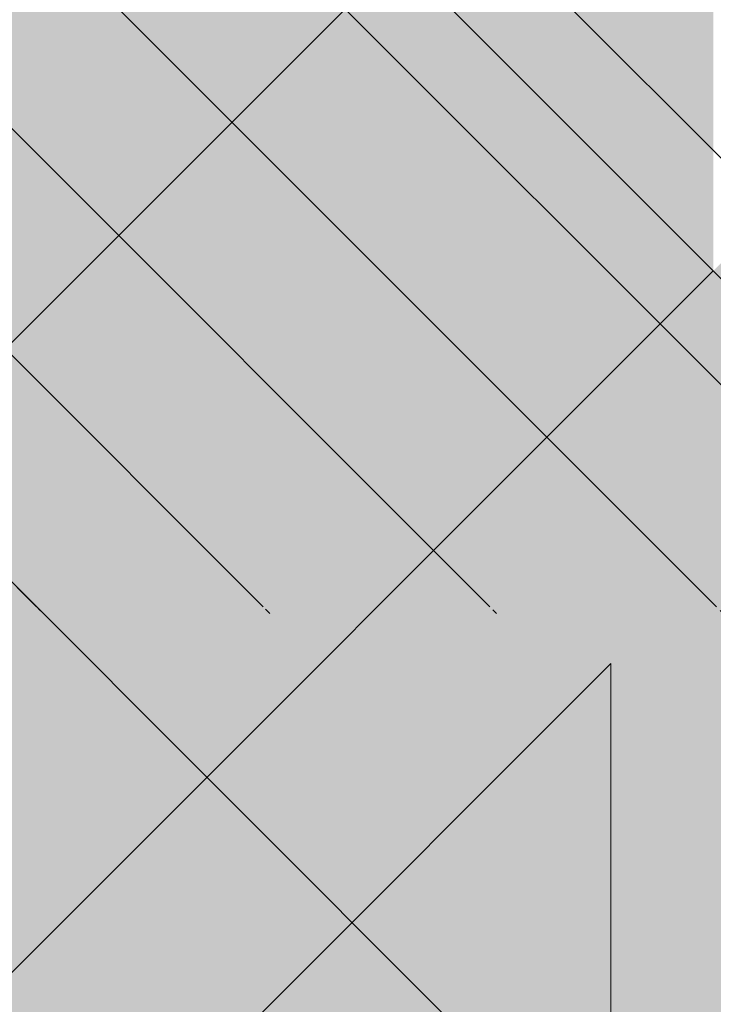
# Model space of a CAD drawing. Units: inches. Extents: x 844 to 2234, y 346 to 1084.
# Tile 80 of 93: x 2002.996 to 2003.858, y 705.162 to 706.386. Entities that reach past the tile are written whole.
import ezdxf

# ---------------------------------------------------------------- set-up
doc = ezdxf.new("R2010")
doc.units = ezdxf.units.IN
doc.header["$MEASUREMENT"] = 0
for name, color, linetype, lineweight in [('A-ANNO-DIMS', 2, 'Continuous', 18), ('furniture', 8, 'Continuous', 18), ('RA-AP-01$0$INT', 35, 'Continuous', 5)]:
    doc.layers.add(name, color=color, linetype=linetype, lineweight=lineweight)
doc.layers.add('RA-AP-01$0$FURN', color=3, linetype='Continuous')
doc.layers.add('RA-AP-01$0$WOOD', color=64, linetype='Continuous')
doc.styles.get("Standard").update_dxf_attribs({"font": 'arial.ttf'})
doc.dimstyles.get("Standard").update_dxf_attribs({"dimtxt": 6, "dimasz": 3, "dimexe": 0.18, "dimexo": 0.0625, "dimgap": 0.09, "dimtad": 0, "dimtih": 1, "dimtoh": 1, "dimdec": 1, "dimzin": 0, "dimdsep": 46, "dimlunit": 3, "dimtxsty": 'Standard', "dimblk": 'ARCHTICK', "dimcen": 0.09, "dimadec": 0, "dimazin": 0, "dimtfac": 1, "dimtdec": 1, "dimtofl": 0, "dimtmove": 0, "dimatfit": 3, "dimfxl": 1, "dimtolj": 1, "dimtzin": 0, "dimarcsym": 0})

# ---------------------------------------------------------------- blocks, each defined once
blk = doc.blocks.new('A$C18D01794')
at = {"layer": 'RA-AP-01$0$INT'}
h = blk.add_hatch(color=256, dxfattribs=at)
h.paths.add_polyline_path([(4.585917135068448, -7.856712009587804), (4.614201406330596, -7.856712009587056), (4.668846067270487, -7.802067348644738), (4.723490728212344, -7.856712009584164), (4.771774999457151, -7.856712009582887), (4.826419660396886, -7.80206734864072), (4.862780050090322, -7.838427738332541), (4.844495778842715, -7.856712009580965), (4.862780050090411, -7.856712009580482), (4.905206456960182, -7.814285602707865), (4.947632863832445, -7.856712009578238), (4.965917135079675, -7.856712009577755), (4.947632863831759, -7.838427738330656), (4.983993253523576, -7.802067348637219), (5.038637914464627, -7.856712009575829), (5.08692218571208, -7.856712009574554), (5.141566846649976, -7.802067348634224), (5.196211507589851, -7.856712009571666), (5.224495778822615, -7.856712009570916), (4.905206456953975, -7.537422687702283)])
h.paths.add_polyline_path([(4.895206456956031, -7.575706958950402), (4.895206456958921, -7.684996280828174), (4.840561796018589, -7.630351619890275)], flags=16)
h.paths.add_polyline_path([(4.915206456955638, -7.575706958949956), (4.969851117895509, -7.630351619887399), (4.915206456957609, -7.684996280827732)], flags=16)
h.paths.add_polyline_path([(4.826419660395175, -7.644493755514321), (4.881064321335613, -7.699138416452331), (4.771774999456703, -7.69913841645522)], flags=16)
h.paths.add_polyline_path([(4.983993253519558, -7.644493755510815), (5.038637914460456, -7.699138416449285), (4.929348592581548, -7.69913841645126)], flags=16)
h.paths.add_polyline_path([(4.881064321336025, -7.719138416452334), (4.826419660397532, -7.773783077393256), (4.771774999457062, -7.719138416455217)], flags=16)
h.paths.add_polyline_path([(4.929348592582019, -7.71913841645126), (5.038637914460982, -7.719138416449284), (4.983993253522945, -7.773783077389749)], flags=16)
h.paths.add_polyline_path([(4.895206456960191, -7.733280552075633), (4.895206456962115, -7.806001331460164), (4.876922185715016, -7.824285602708492), (4.840561796021581, -7.787925213016675)], flags=16)
h.paths.add_polyline_path([(4.915206456958487, -7.733280552075187), (4.969851117899527, -7.787925213013798), (4.933490728206909, -7.824285602708034), (4.9152064569598, -7.806001331461736)], flags=16)
h.paths.add_polyline_path([(4.757632863832376, -7.733280552079264), (4.812277524772842, -7.787925213017304), (4.757632863834348, -7.842569873958233)], flags=16)
h.paths.add_polyline_path([(4.737632863832376, -7.73328055207979), (4.737632863834348, -7.842569873958701), (4.682988202893906, -7.787925213020692)], flags=16)
h.paths.add_polyline_path([(5.05278005008503, -7.733280552072701), (5.052780050087917, -7.842569873951664), (4.998135389146995, -7.787925213013169)], flags=16)
h.paths.add_polyline_path([(5.072780050085024, -7.733280552072333), (5.127424711025931, -7.787925213010806), (5.072780050087916, -7.842569873951244)], flags=16)
h.paths.add_polyline_path([(4.935917135072783, -7.506712009583784), (5.255206456948811, -7.826001331459767), (5.255206456948932, -7.797717060211899), (5.200561796010279, -7.743072399273238), (5.255206456949403, -7.688427738334128), (5.25520645694961, -7.640143467086677), (5.200561796009787, -7.585498806146837), (5.236922185702417, -7.549138416454212), (5.255206456949919, -7.56742268770172), (5.255206456949998, -7.549138416454178), (5.212780050078687, -7.506712009583814), (5.25520645695036, -7.464285602712145), (5.255206456950438, -7.446001331464763), (5.236922185702424, -7.464285602712779), (5.200561796009796, -7.427925213020149), (5.255206456950753, -7.373280552079203), (5.25520645695096, -7.324996280834394), (5.200561796010322, -7.270351619893748), (5.255206456951428, -7.215706958952649), (5.255206456951547, -7.187422687705071)])
h.paths.add_polyline_path([(5.042988202883395, -7.42792521302065), (5.097632863823085, -7.373280552080975), (5.097632863822622, -7.482569873959883)], flags=16)
h.paths.add_polyline_path([(5.028846067259663, -7.442067348644384), (5.083490728198774, -7.496712009583504), (4.974201406321001, -7.496712009583035)], flags=16)
h.paths.add_polyline_path([(5.117632863823087, -7.37328055208089), (5.172277524762331, -7.42792521302015), (5.11763286382262, -7.482569873959851)], flags=16)
h.paths.add_polyline_path([(5.08349072819877, -7.516712009582191), (5.028846067259652, -7.571356670521302), (4.974201406320998, -7.516712009582638)], flags=16)
h.paths.add_polyline_path([(5.131774999446817, -7.35913841645716), (5.186419660386065, -7.413783077396415), (5.241064321325782, -7.359138416456712)], flags=17)
h.paths.add_polyline_path([(5.131774999446228, -7.496712009583703), (5.186419660386065, -7.442067348643883), (5.222780050079488, -7.478427738337313), (5.204495778832781, -7.496712009584014)], flags=16)
h.paths.add_polyline_path([(5.097632863822613, -7.530854145205813), (5.097632863823061, -7.640143467084723), (5.042988202883383, -7.585498806145032)], flags=16)
h.paths.add_polyline_path([(5.131774999446899, -7.339138416457162), (5.241064321325809, -7.339138416456712), (5.186419660386591, -7.284493755517479)], flags=17)
h.paths.add_polyline_path([(5.131774999446226, -7.516712009581999), (5.204495778830767, -7.516712009581702), (5.22278005007868, -7.534996280829206), (5.186419660386049, -7.571356670521828)], flags=16)
h.paths.add_polyline_path([(5.11763286382262, -7.530854145205852), (5.17227752476232, -7.585498806145562), (5.117632863823064, -7.64014346708481)], flags=16)
h.paths.add_polyline_path([(5.186419660386069, -7.599640941770585), (5.241064321325754, -7.654285602710281), (5.131774999446791, -7.654285602709814)], flags=16)
h.paths.add_polyline_path([(5.131774999446872, -7.674285602709813), (5.24106432132578, -7.674285602710282), (5.186419660386554, -7.728930263649504)], flags=16)
h.paths.add_polyline_path([(5.255206456951811, -7.126001331467467), (5.255206456951895, -7.106712009588038), (4.555206456956052, -7.106712009588038), (4.555206456956136, -7.12600133146746), (4.905206456953973, -7.476001331465289)])
h.paths.add_polyline_path([(4.983993253513404, -7.368930263651977), (4.92934859257295, -7.314285602713969), (5.03863791445186, -7.314285602711063)], flags=16)
h.paths.add_polyline_path([(4.969851117889988, -7.383072399276016), (4.915206456952556, -7.437717060215906), (4.915206456949648, -7.328427738338133)], flags=16)
h.paths.add_polyline_path([(4.929348592572535, -7.294285602713971), (4.983993253511019, -7.239640941773039), (5.038637914451496, -7.294285602711065)], flags=16)
h.paths.add_polyline_path([(5.052780050074912, -7.280143467087016), (4.998135389134438, -7.225498806148989), (5.052780050072919, -7.170854145208052)], flags=16)
h.paths.add_polyline_path([(5.07278005007491, -7.280143467086489), (5.072780050072918, -7.170854145207579), (5.127424711013374, -7.225498806145578)], flags=16)
h.paths.add_polyline_path([(4.89520645695295, -7.437717060216355), (4.840561796013067, -7.383072399278919), (4.895206456950961, -7.328427738338582)], flags=16)
h.paths.add_polyline_path([(4.915206456948365, -7.280143467090674), (4.915206456946434, -7.207422687704125), (4.933490728192729, -7.18913841645701), (4.969851117886972, -7.225498806149623)], flags=16)
h.paths.add_polyline_path([(4.881064321327021, -7.314285602715054), (4.82641966038902, -7.368930263655506), (4.771774999448108, -7.314285602717047)], flags=16)
h.paths.add_polyline_path([(4.895206456950073, -7.280143467091125), (4.840561796009022, -7.225498806152518), (4.876922185700835, -7.18913841645908), (4.895206456948749, -7.207422687706589)], flags=16)
h.paths.add_polyline_path([(4.983993253510392, -7.211356670525576), (4.947632863816944, -7.174996280833758), (4.965917135064043, -7.156712009585847), (5.038637914448995, -7.156712009584522)], flags=16)
h.paths.add_polyline_path([(4.881064321326543, -7.294285602715056), (4.771774999447578, -7.294285602717046), (4.826419660385607, -7.239640941776569)], flags=16)
h.paths.add_polyline_path([(4.905206456946447, -7.19913841645844), (4.862780050074785, -7.156712009587725), (4.947632863816685, -7.156712009586302)], flags=16)
h.paths.add_polyline_path([(5.14156684663679, -7.211356670521528), (5.086922185696452, -7.156712009583639), (5.196211507574223, -7.156712009581651)], flags=16)
h.paths.add_polyline_path([(4.8264196603837, -7.211356670529104), (4.771774999442643, -7.156712009590501), (4.8444957788276, -7.156712009588568), (4.862780050075511, -7.17499628083566)], flags=16)
h.paths.add_polyline_path([(4.812277524760289, -7.225498806153156), (4.757632863822258, -7.28014346709363), (4.757632863819352, -7.170854145214669)], flags=16)
h.paths.add_polyline_path([(4.73763286382226, -7.280143467093997), (4.682988202881349, -7.22549880615554), (4.737632863819352, -7.170854145215086)], flags=16)
h.paths.add_polyline_path([(4.723490728195188, -7.156712009591787), (4.668846067257299, -7.211356670532127), (4.614201406317417, -7.156712009594693)], flags=16)
h.paths.add_polyline_path([(4.597632863829262, -7.506712009583814), (4.555206456957951, -7.54913841645418), (4.555206456958029, -7.56742268770172), (4.573490728205535, -7.549138416454212), (4.609851117898167, -7.585498806146839), (4.555206456958338, -7.640143467086675), (4.555206456958546, -7.688427738334125), (4.60985111789767, -7.743072399273238), (4.555206456959015, -7.797717060211899), (4.555206456959138, -7.826001331459767), (4.874495778835167, -7.506712009583786), (4.5552064569564, -7.187422687705062), (4.555206456956523, -7.215706958952644), (4.609851117897629, -7.270351619893746), (4.555206456956988, -7.324996280834396), (4.555206456957198, -7.373280552079195), (4.609851117898153, -7.427925213020147), (4.573490728205528, -7.464285602712779), (4.555206456957507, -7.446001331464756), (4.555206456957585, -7.464285602712143)])
h.paths.add_polyline_path([(4.712780050085332, -7.482569873959882), (4.712780050084863, -7.373280552080972), (4.767424711024555, -7.42792521302065)], flags=16)
h.paths.add_polyline_path([(4.726922185709173, -7.496712009583504), (4.781566846648288, -7.442067348644384), (4.836211507586949, -7.496712009583033)], flags=16)
h.paths.add_polyline_path([(4.692780050085327, -7.482569873959851), (4.638135389145619, -7.427925213020149), (4.692780050084865, -7.373280552080892)], flags=16)
h.paths.add_polyline_path([(4.726922185709182, -7.516712009582191), (4.836211507586949, -7.51671200958264), (4.7815668466483, -7.571356670521304)], flags=16)
h.paths.add_polyline_path([(4.678637914461726, -7.496712009583706), (4.605917135075169, -7.496712009584014), (4.587632863828464, -7.478427738337311), (4.623993253521887, -7.442067348643881)], flags=16)
h.paths.add_polyline_path([(4.712780050085336, -7.530854145205816), (4.767424711024568, -7.585498806145034), (4.71278005008489, -7.640143467084724)], flags=16)
h.paths.add_polyline_path([(4.678637914461726, -7.516712009582001), (4.623993253521899, -7.571356670521829), (4.587632863829271, -7.534996280829206), (4.605917135077185, -7.5167120095817)], flags=16)
h.paths.add_polyline_path([(4.692780050085336, -7.530854145205848), (4.692780050084889, -7.64014346708481), (4.638135389145632, -7.585498806145562)], flags=16)
h.paths.add_polyline_path([(4.623993253521885, -7.413783077396415), (4.678637914461131, -7.359138416457161), (4.56934859258217, -7.359138416456712)], flags=17)
h.paths.add_polyline_path([(4.623993253521901, -7.599640941770568), (4.678637914461158, -7.654285602709814), (4.569348592582195, -7.654285602710281)], flags=16)
h.paths.add_polyline_path([(4.678637914461051, -7.339138416457162), (4.623993253521361, -7.284493755517479), (4.569348592582143, -7.339138416456712)], flags=17)
h.paths.add_polyline_path([(4.678637914461076, -7.674285602709813), (4.623993253521399, -7.728930263649504), (4.569348592582167, -7.674285602710281)], flags=16)
h = blk.add_hatch(color=256, dxfattribs=at)
h.paths.add_polyline_path([(4.905206456954232, -7.537422687702028), (4.874495778835232, -7.506712009583718), (4.555206456959138, -7.826001331459766), (4.555206456959269, -7.856712009588616), (4.585917135068449, -7.856712009587804)])
h.paths.add_polyline_path([(4.935917135072152, -7.506712009583152), (4.905206456953497, -7.537422687701806), (5.224495778822614, -7.856712009570917), (5.255206456948681, -7.856712009570104), (5.255206456948813, -7.826001331459768)])
h.paths.add_polyline_path([(5.255206456951549, -7.18742268770507), (5.255206456951813, -7.126001331467461), (4.905206456953563, -7.476001331465701), (4.935917135072559, -7.506712009584006)])
h.paths.add_polyline_path([(4.874495778835167, -7.506712009583785), (4.905206456953818, -7.476001331465132), (4.555206456956135, -7.126001331467458), (4.555206456956399, -7.187422687705064)])
h = blk.add_hatch(color=256, dxfattribs=at)
h.paths.add_polyline_path([(4.89520645695096, -7.328427738338579), (4.840561796013068, -7.383072399278921), (4.89520645695295, -7.437717060216353)])
h.paths.add_polyline_path([(4.915206456952557, -7.437717060215907), (4.969851117889986, -7.383072399276024), (4.915206456949648, -7.328427738338133)])
h.paths.add_polyline_path([(4.929348592572952, -7.31428560271397), (4.983993253513403, -7.368930263651974), (5.038637914451863, -7.314285602711064)])
h.paths.add_polyline_path([(5.038637914451498, -7.294285602711065), (4.983993253511018, -7.239640941773039), (4.929348592572535, -7.294285602713969)])
h.paths.add_polyline_path([(4.969851117886971, -7.225498806149624), (4.93349072819273, -7.189138416457011), (4.915206456946433, -7.207422687704124), (4.915206456948367, -7.280143467090678)])
h.paths.add_polyline_path([(4.965917135064045, -7.156712009585847), (4.947632863816945, -7.17499628083376), (4.983993253510389, -7.211356670525573), (5.038637914448995, -7.156712009584522)])
h.paths.add_polyline_path([(4.998135389134439, -7.22549880614899), (5.05278005007491, -7.280143467087016), (5.052780050072921, -7.170854145208054)])
h.paths.add_polyline_path([(5.072780050074911, -7.28014346708649), (5.127424711013374, -7.225498806145579), (5.072780050072921, -7.170854145207581)])
h.paths.add_polyline_path([(5.196211507574225, -7.156712009581651), (5.08692218569645, -7.156712009583639), (5.141566846636789, -7.211356670521529)])
h.paths.add_polyline_path([(4.862780050074782, -7.156712009587723), (4.90520645694645, -7.199138416458444), (4.94763286381669, -7.156712009586302)])
h.paths.add_polyline_path([(4.895206456950073, -7.280143467091126), (4.895206456948746, -7.207422687706587), (4.876922185700836, -7.189138416459078), (4.840561796009025, -7.225498806152521)])
h.paths.add_polyline_path([(4.826419660385605, -7.239640941776569), (4.771774999447577, -7.294285602717049), (4.881064321326541, -7.294285602715055)])
h.paths.add_polyline_path([(4.771774999448108, -7.314285602717046), (4.82641966038902, -7.368930263655505), (4.88106432132702, -7.314285602715054)])
h.paths.add_polyline_path([(4.757632863822258, -7.280143467093631), (4.812277524760285, -7.225498806153153), (4.757632863819352, -7.170854145214668)])
h.paths.add_polyline_path([(4.862780050075512, -7.17499628083566), (4.844495778827599, -7.156712009588567), (4.771774999442647, -7.156712009590504), (4.8264196603837, -7.211356670529104)])
h.paths.add_polyline_path([(4.682988202881349, -7.225498806155537), (4.737632863822258, -7.280143467093997), (4.737632863819352, -7.170854145215087)])
h.paths.add_polyline_path([(4.723490728195189, -7.156712009591783), (4.614201406317418, -7.156712009594692), (4.668846067257298, -7.211356670532127)])
h = blk.add_hatch(color=256, dxfattribs=at)
h.paths.add_polyline_path([(4.874495778835231, -7.506712009583718), (4.905206456953751, -7.537422687701551), (4.905206456953581, -7.506712009583548)])
h.paths.add_polyline_path([(4.905206456953409, -7.476001331465546), (4.905206456953583, -7.506712009583546), (4.935917135071927, -7.506712009583376)])
for p, q in [((4.905206456953975, -7.476001331465289), (4.555206456956136, -7.12600133146746)), ((4.905206456953975, -7.476001331465289), (5.255206456951811, -7.126001331467465)), ((4.935917135072783, -7.506712009583784), (5.255206456951548, -7.187422687705069)), ((4.915206456949648, -7.328427738338135), (4.915206456952556, -7.437717060215906)), ((4.915206456952556, -7.437717060215906), (4.969851117889986, -7.383072399276024)), ((4.935917135071927, -7.506712009583376), (4.905206456953407, -7.476001331465544))]:
    blk.add_line(p, q, dxfattribs=at)
blk = doc.blocks.new('A$C32926AE1')
at = {"layer": 'RA-AP-01$0$FURN'}
h = blk.add_hatch(dxfattribs=at)
h.set_pattern_fill('ANSI31', color=256, scale=0.1, style=0)
h.set_pattern_definition([(45, (0, 0), (-0.0088388347648318, 0.0088388347648318), [])])
edge = h.paths.add_edge_path(flags=16)
edge.add_arc((4.904771284329206, 4.246793130718756), 0.2603971832811541, 75.22398030683196, 104.7760196931204)
edge.add_arc((4.904771284329206, 4.246793130718756), 0.2603971832811541, 75.223980306832, 104.77601969312039, ccw=False)
edge = h.paths.add_edge_path(flags=16)
edge.add_arc((4.904771284329206, 4.067062675376612), 0.2603971832811541, 255.2239803068796, 284.776019693168)
edge.add_arc((4.904771284329206, 4.067062675376612), 0.2603971832811541, 255.22398030687958, 284.77601969316805, ccw=False)
edge = h.paths.add_edge_path(flags=0)
edge.add_arc((4.904771284329206, 4.067062675376612), 0.2603971832811541, 255.2239803068796, 284.776019693168)
edge.add_arc((4.904771284329206, 4.067062675376612), 0.2603971832811541, 255.22398030687958, 284.77601969316805, ccw=False)
edge = h.paths.add_edge_path(flags=0)
edge.add_arc((4.904771284329206, 4.067062675376612), 0.2603971832811541, 255.2239803068796, 284.776019693168)
edge.add_arc((4.904771284329206, 4.067062675376612), 0.2603971832811541, 255.22398030687958, 284.77601969316805, ccw=False)
edge = h.paths.add_edge_path()
edge.add_arc((4.604388392048174, 4.588829985554312), 0.1599999999999918, 342.3781640246255, 354.4317409793762)
edge.add_arc((5.090145208887507, 4.43216705527679), 0.3503971832811637, 162.0091218307731, 180.3186872093483)
edge.add_arc((5.205154176610243, 4.588829985554953), 0.1599999999999917, 185.5682590208461, 197.6218359767349)
edge.add_arc((4.904771284329229, 4.246793130718735), 0.3503971832811761, 72.00912183053516, 107.9908781690354)
edge.add_arc((9.535952835716557, 4.28682295566602), 4.798342501046485, 178.2875002453811, 181.5576802719453)
edge.add_arc((4.719397359771122, 4.43216705527679), 0.3503971832811637, 359.6813127906516, 377.9908781692269)
edge.add_arc((9.535967292294904, 4.286822350292874), 4.778371420254705, 178.2965938931842, 181.5667745797229)
edge.add_arc((4.719397359771122, 4.43216705527679), 0.3303971832811637, 359.6813127906516, 377.9908781692269)
edge.add_arc((0.2735752763637294, 4.286822350292874), 4.7783714202547, 358.4332254202771, 361.7034061068158)
edge.add_arc((5.061434214606998, 4.732549947558029), 0.1600000000000254, 252.3781640250584, 264.4317409792362)
edge.add_arc((4.748108354051257, 4.732549947558012), 0.1600000000000541, 275.5682590208426, 287.6218359759532)
edge.add_arc((4.604388392048115, 4.588829985554317), 0.1800000000000505, 342.3567572500182, 349.3735009646207)
edge.add_arc((5.205154176610254, 4.588829985554976), 0.1800000000000069, 190.6264990356027, 197.6432427513933)
edge.add_arc((5.061434214607106, 4.732549947558013), 0.1800000000000424, 252.3567572496606, 259.3735009644582)
edge.add_arc((4.904771284329208, 4.246793130718737), 0.3303971832811676, 71.99844483668534, 108.0015551637021)
edge.add_arc((4.748108354051414, 4.732549947558045), 0.1800000000000547, 280.6264990355479, 287.6432427495938)
edge.add_arc((5.090145208887514, 4.432167055276789), 0.2803971832811691, 162.8706300666893, 180.816523289902)
edge.add_arc((4.719397359771136, 4.432167055276689), 0.2803971832811534, 359.183476710103, 377.1293699333214)
edge.add_arc((4.904771284329222, 4.246793130718737), 0.2803971832811769, 72.87063006672916, 107.1293699332334)
edge.add_arc((5.090145208887522, 4.432167055276788), 0.2603971832811776, 165.2239803068007, 180.9953123810312)
edge.add_arc((4.719397359771141, 4.432167055276699), 0.2603971832811458, 359.0046876189768, 374.7760196932087)
edge.add_arc((5.090145208887507, 4.43216705527679), 0.3303971832811637, 162.0091218307731, 180.3186872093483)
edge.add_arc((9.53595427642584, 4.285015535491528), 4.728345371032053, 178.265043920078, 181.5679956281801)
edge.add_arc((0.2735882922327999, 4.285015535491582), 4.728345371032045, 358.4320043718193, 361.7349560799204)
edge.add_arc((9.535953591267507, 4.284458026472751), 4.708343996644348, 178.2573054306777, 181.5704995759608)
edge.add_arc((0.273588977391114, 4.284458026472785), 4.708343996644358, 358.4295004240388, 361.7426945693213)
edge.add_arc((0.2735889773911131, 4.029397779622582), 4.708343996644359, 358.2573054306787, 361.5704995759613)
edge.add_arc((9.535953591267518, 4.029397779622618), 4.708343996644359, 178.4295004240391, 181.7426945693223)
edge.add_arc((0.2735882922327901, 4.028840270603786), 4.728345371032054, 358.2650439200796, 361.5679956281808)
edge.add_arc((9.53595427642584, 4.028840270603841), 4.728345371032054, 178.4320043718199, 181.7349560799219)
edge.add_arc((0.2735752763637302, 4.027033455802493), 4.778371420254699, 358.2965938931842, 361.5667745797229)
edge.add_arc((4.719397359771122, 3.881688750818578), 0.3303971832811637, 342.0091218307731, 360.3186872093484)
edge.add_arc((5.090145208887507, 3.881688750818578), 0.3303971832811637, 179.6813127906516, 197.9908781692269)
edge.add_arc((9.535967292294904, 4.027033455802493), 4.778371420254705, 178.433225420277, 181.7034061068158)
edge.add_arc((4.719397359771122, 3.881688750818578), 0.3503971832811637, 342.0091218307731, 360.3186872093484)
edge.add_arc((9.53595283571655, 4.027032850429349), 4.79834250104648, 178.4423197280546, 181.7124997546188)
edge.add_arc((4.719397359771141, 3.881688750818669), 0.2603971832811458, 345.2239803067913, 360.9953123810232)
edge.add_arc((5.090145208887522, 3.88168875081858), 0.2603971832811776, 179.0046876189687, 194.7760196931993)
edge.add_arc((4.904771284329222, 4.067062675376631), 0.2803971832811769, 252.8706300667665, 287.1293699332708)
edge.add_arc((4.719397359771136, 3.881688750818678), 0.2803971832811534, 342.8706300666787, 360.8165232898969)
edge.add_arc((5.090145208887514, 3.881688750818579), 0.2803971832811691, 179.183476710098, 197.1293699333106)
edge.add_arc((4.748108354051414, 3.581305858537323), 0.1800000000000547, 72.3567572504062, 79.37350096445199)
edge.add_arc((4.904771284329208, 4.067062675376631), 0.3303971832811676, 251.9984448362979, 288.0015551633146)
edge.add_arc((5.061434214607106, 3.581305858537355), 0.1800000000000424, 100.6264990355418, 107.6432427503394)
edge.add_arc((5.205154176610254, 3.725025820540392), 0.1800000000000069, 162.3567572486066, 169.3735009643972)
edge.add_arc((4.604388392048115, 3.725025820541051), 0.1800000000000505, 10.62649903537925, 17.64324274998182)
edge.add_arc((4.748108354051257, 3.581305858537356), 0.1600000000000541, 72.37816402404681, 84.43174097915735)
edge.add_arc((4.904771284329229, 4.067062675376632), 0.3503971832811761, 252.0091218309645, 287.9908781694648)
edge.add_arc((5.061434214606998, 3.581305858537339), 0.1600000000000254, 95.56825902076373, 107.6218359749416)
edge.add_arc((5.205154176610243, 3.725025820540414), 0.1599999999999917, 162.3781640232651, 174.4317409791539)
edge.add_arc((5.090145208887507, 3.881688750818578), 0.3503971832811637, 179.6813127906516, 197.9908781692269)
edge.add_arc((4.604388392048174, 3.725025820541056), 0.1599999999999918, 5.568259020623824, 17.62183597537444)
edge.add_arc((0.2735897329420762, 4.28682295566602), 4.798342501046482, 358.4423197280547, 361.7124997546188)
edge.add_arc((0.2735897329420691, 4.027032850429348), 4.798342501046489, 358.2875002453812, 361.5576802719453)
at = {"layer": 'RA-AP-01$0$WOOD'}
h = blk.add_hatch(color=256, dxfattribs=at)
h.dxf.hatch_style = 1
h.paths.add_polyline_path([(5.157430609644524, 4.573483066760929, -0.1009492694046607), (5.155401577623758, 4.593365984175333, -0.1842662638101597), (5.172249623284174, 4.638795604568598, 0.2056608120311276), (5.179560981299304, 4.661316324430096, 0.3614336704623542), (5.134352340494423, 4.706524965234944, 0.2056608120311297), (5.111831620632933, 4.699213607219793, -0.1842662638101113), (5.066402000239693, 4.682365561559342, -0.1055311479399994), (5.045656153913092, 4.68467289944697, 0.1567636581983829), (4.763886414745334, 4.684672899446966, -0.1055311479399895), (4.743140568418733, 4.68236556155934, -0.1842662638100833), (4.6977109480255, 4.69921360721979, 0.2056608120302612), (4.675190228164109, 4.706524965234949, 0.3614336704708441), (4.629981587358889, 4.66131632442871, 0.2056608120245944), (4.637292945374126, 4.638795604567974, -0.1842662638101024), (4.654140991034615, 4.59336598417475, -0.1009492694055169), (4.652111959013835, 4.573483066760181, 0.021410119221476), (4.629748025606143, 4.156712009541676, 0.0214101192214795), (4.652111959013809, 3.739940952323101, -0.1009492694059586), (4.654140991034615, 3.720058034908448, -0.1842662638100975), (4.637292945374126, 3.674628414515226, 0.2056608120245705), (4.629981587358889, 3.652107694654492, 0.3614336704708879), (4.675190228164113, 3.606899053848249, 0.2056608120302384), (4.697710948025501, 3.614210411863408, -0.1842662638100995), (4.743140568418738, 3.63105845752386, -0.1055311479402541), (4.763886414745388, 3.628751119636215, 0.1567636581983776), (5.045656153913137, 3.628751119636244, -0.1055311479397538), (5.066402000239692, 3.631058457523857, -0.1842662638101067), (5.111831620632931, 3.614210411863407, 0.2056608120310924), (5.134352340494417, 3.606899053848256, 0.3614336704624001), (5.179560981299307, 3.652107694653103, 0.2056608120311314), (5.172249623284175, 3.6746284145146, -0.1842662638101402), (5.155401577623758, 3.72005803490786, -0.1009492694051366), (5.15743060964455, 3.739940952322354, 0.0214101192215073), (5.179794543052287, 4.156712009541468, 0.0214101192215252)])
h.paths.add_polyline_path([(4.639748609479751, 4.156712009541513, 0.0213537860821624), (4.661970494867118, 3.741887061152232, -0.094075836301374), (4.664143710413708, 3.7196126951003, -0.1824818158568985), (4.644813765429836, 3.668037719127816, 0.2056608120245319), (4.639939526753007, 3.653023905887301, 0.3614336704710246), (4.676106439397173, 3.616856993242342, 0.2056608120302234), (4.691120252638095, 3.621731231919122, -0.1824818158602558), (4.742695228611606, 3.641061176902986, -0.1029891339458722), (4.766991894714349, 3.638256818950944, 0.156709409989566), (5.042550673941472, 3.638256818950105, -0.102989133958497), (5.066847340047078, 3.641061176902949, -0.1824818158594995), (5.118422316020358, 3.621731231919103, 0.2056608120311416), (5.133436129261316, 3.616856993242346, 0.3614336704621468), (5.169603041905217, 3.653023905886178, 0.2056608120310986), (5.164728803228477, 3.668037719127177, -0.1824818158565612), (5.145398858244737, 3.719612695099578, -0.0940758363009313), (5.147572073791232, 3.741887061151398, 0.0213537860822023), (5.169793959178681, 4.156712009541451, 0.0213537860822226), (5.147572073791203, 4.571536957931898, -0.0940758363005034), (5.145398858244737, 4.59381132398362, -0.1824818158565587), (5.164728803228476, 4.645386299956021, 0.2056608120311045), (5.169603041905216, 4.66040011319702, 0.3614336704621845), (5.133436129261313, 4.696567025840856, 0.2056608120310773), (5.118422316020359, 4.691692787164098, -0.182481815859508), (5.066847340047078, 4.67236284218025, -0.1029891339584606), (5.04255067394148, 4.675167200133092, 0.156709409989566), (4.766991894714357, 4.675167200132257, -0.1029891339458842), (4.742695228611611, 4.672362842180213, -0.1824818158602725), (4.691120252638095, 4.691692787164077, 0.2056608120302152), (4.676106439397174, 4.696567025840858, 0.3614336704710363), (4.639939526753005, 4.660400113195899, 0.2056608120245495), (4.644813765429837, 4.645386299955384, -0.1824818158568934), (4.664143710413708, 4.593811323982902, -0.0940758363009187), (4.661970494867149, 4.571536957931074, 0.021353786082177)], flags=16)
h.paths.add_polyline_path([(5.129794543052235, 4.432167055276933, -0.0141661062790638), (5.130152669293814, 4.156927903047693, -0.0141661062790647), (5.129794543052234, 3.881688750818433, -0.0785247771143638), (5.10979738006795, 3.755143611847103, 0.0945969212073497), (5.105408519571111, 3.717898134952927, 0.1043170707844957), (5.116074640131521, 3.670385395016088, 0.1043170707864965), (5.068561900193738, 3.681051515576561, 0.09459692119553), (5.031316423304057, 3.676662655080835, -0.1580239521427272), (4.778226145355827, 3.676662655080367, 0.0945969211986668), (4.740980668464973, 3.681051515576592, 0.1043170707882822), (4.693467928526415, 3.670385395015844, 0.1043170707867916), (4.704134049087309, 3.717898134953662, 0.0945969211972894), (4.69974518859162, 3.755143611844042, -0.0785247771163196), (4.679748025606343, 3.881688750818406, -0.0141661062790663), (4.679389899364763, 4.156927903047693, -0.0141661062790672), (4.679748025606343, 4.432167055276998, -0.0785247771163064), (4.699745188591625, 4.55871219425134, 0.094596921197333), (4.704134049087308, 4.595957671141738, 0.1043170707867205), (4.693467928526416, 4.643470411079523, 0.1043170707882628), (4.740980668464965, 4.632804290518776, 0.0945969211988114), (4.778226145355874, 4.637193151015016, -0.158023952142669), (5.031316423304015, 4.637193151014546, 0.0945969211956361), (5.068561900193736, 4.632804290518806, 0.1043170707864979), (5.11607464013152, 4.643470411079278, 0.1043170707844617), (5.105408519571112, 4.595957671142455, 0.0945969212074597), (5.109797380067959, 4.558712194248236, -0.0785247771143467)], flags=0)
h.paths.add_polyline_path([(5.119794532311105, 4.432259799204851, -0.0142000800617244), (5.120156169157484, 4.156927903047701, -0.0142000800617277), (5.119794532311105, 3.881596006890482, -0.0784894509520253), (5.100273383573699, 3.758192358677797, 0.0940138827242913), (5.095413455884425, 3.717477693979438, 0.0606271852308753), (5.099615656341024, 3.686844378806616, 0.0606271852322524), (5.068982341167493, 3.691046579263239, 0.0940138827010453), (5.028267676478798, 3.686186651576848, -0.1580706864508061), (4.781274892180912, 3.686186651576435, 0.0940138827026903), (4.740560227491556, 3.691046579263279, 0.0606271852339895), (4.709926912317155, 3.686844378806508, 0.0606271852329405), (4.714129112773991, 3.717477693980356, 0.094013882701304), (4.709269185087677, 3.758192358669163, -0.0784894509577193), (4.689748036347473, 3.881596006890469, -0.014200080061729), (4.689386399501094, 4.156927903047709, -0.0142000800617217), (4.689748036347473, 4.432259799204808, -0.078489450957724), (4.709269185087651, 4.555663447426125, 0.0940138827014585), (4.714129112773992, 4.596378112114996, 0.0606271852329731), (4.709926912317154, 4.62701142728886, 0.0606271852340196), (4.74056022749157, 4.622809226832087, 0.0940138827024997), (4.781274892180847, 4.627669154518912, -0.1580706864508359), (5.028267676478777, 4.627669154518526, 0.0940138827010946), (5.068982341167492, 4.622809226832129, 0.060627185232254), (5.099615656341024, 4.627011427288751, 0.0606271852308727), (5.095413455884425, 4.59637811211593, 0.0940138827241088), (5.100273383573675, 4.555663447417647, -0.0784894509520978)], flags=0)
h.paths.add_polyline_path([(5.06978912287499, 4.430218106756144, -0.014241683694547), (5.070173729147532, 4.156927903047672, -0.0142416836945458), (5.06978912287499, 3.883637699339223, -0.0800609523125196), (5.052662118612511, 3.773463122773442, 0.0526421978001116), (5.04590916754064, 3.740550867606997, 0.0526421977992423), (5.012996912374707, 3.73379791653534, -0.1583028414718258), (4.796545656286308, 3.73379791653451, 0.0526421978034211), (4.763633401117837, 3.740550867607021, 0.0526421978018622), (4.756880450045755, 3.773463122774558, -0.0800609523117106), (4.739753445783639, 3.883637699339268, -0.0142416836945435), (4.739368839511098, 4.156927903047671, -0.0142416836945477), (4.739753445783639, 4.430218106756155, -0.0800609523116345), (4.75688045004574, 4.540392683320762, 0.052642197801941), (4.763633401117837, 4.573304938488346, 0.0526421978035071), (4.796545656286361, 4.580057889560873, -0.1583028414717561), (5.012996912374669, 4.580057889560039, 0.0526421977993048), (5.04590916754064, 4.57330493848837, 0.0526421978002057), (5.052662118612529, 4.540392683321868, -0.080060952312477)], flags=0)
h.paths.add_polyline_path([(5.049789715110557, 4.43038092723357, -0.0143097550741839), (5.05018085590259, 4.156927903047715, -0.0143097550741854), (5.049789715110558, 3.883474878861827, -0.0800685599149176), (5.03362098255317, 3.779581877367999, 0.0306258898956367), (5.028241146483733, 3.758218888663947, 0.0306258898977031), (5.006878157778253, 3.75283905259408, -0.1583983521624096), (4.802664410878162, 3.752839052594731, 0.0306258898946014), (4.781301422174808, 3.758218888663924, 0.0306258898967912), (4.775921586105202, 3.779581877368794, -0.080068559914251), (4.759752853548071, 3.883474878861786, -0.0143097550741854), (4.759361712756037, 4.156927903047671, -0.0143097550741854), (4.759752853548071, 4.430380927233557, -0.0800685599142479), (4.775921586105193, 4.534273928726546, 0.0306258898968306), (4.781301422174808, 4.555636917431444, 0.0306258898945754), (4.802664410878143, 4.561016753500631, -0.1583983521624168), (5.006878157778244, 4.561016753501291, 0.0306258898977177), (5.028241146483733, 4.555636917431421, 0.0306258898958182), (5.03362098255321, 4.534273928727244, -0.080068559914796)], flags=0)
h.paths.add_polyline_path([(4.999766070382627, 4.428171244713864, -0.0143443147609634), (5.000198441819402, 4.156927903047689, -0.0143443147609612), (4.999766070382627, 3.885684561381556, -0.0784641635803329), (4.987356730658798, 3.799103304488872, -0.1506053783831347), (4.822185837999821, 3.79910330448882, -0.0784641635803318), (4.809776498276007, 3.885684561381509, -0.014344314760963), (4.809344126839227, 4.156927903047677, -0.0143443147609645), (4.809776498276007, 4.428171244713873, -0.0784641635803192), (4.822185837999822, 4.514752501606549, -0.1506053783831338), (4.987356730658798, 4.514752501606494, -0.078464163580285)], flags=0)
h.paths.add_polyline_path([(4.979755254238824, 4.42764379880488, -0.0143772539198268), (4.980205517789977, 4.156927903047693, -0.0143772539198275), (4.979755254238824, 3.886212007290489, -0.0689242507424422), (4.971183264704897, 3.815276770442801, -0.1296645318904179), (4.838359303953726, 3.815276770442746, -0.0689242507424186), (4.829787314419809, 3.886212007290419, -0.0143772539198292), (4.829337050868653, 4.156927903047653, -0.0143772539198325), (4.829787314419809, 4.427643798804946, -0.0689242507424211), (4.838359303953725, 4.498579035652621, -0.1296645318904187), (4.971183264704897, 4.498579035652565, -0.0689242507424401)], flags=0)
h = blk.add_hatch(color=256, dxfattribs=at)
h.dxf.hatch_style = 1
h.paths.add_polyline_path([(5.145398858244737, 4.59381132398362, -0.1824818158565616), (5.164728803228476, 4.645386299956021, 0.2056608120311045), (5.169603041905216, 4.66040011319702, 0.3614336704621845), (5.133436129261313, 4.696567025840856, 0.2056608120310773), (5.118422316020359, 4.691692787164098, -0.182481815859508), (5.066847340047078, 4.67236284218025, -0.1029891339584606), (5.04255067394148, 4.675167200133092, 0.156709409989566), (4.766991894714357, 4.675167200132257, -0.1029891339458842), (4.742695228611611, 4.672362842180213, -0.1824818158602725), (4.691120252638095, 4.691692787164077, 0.2056608120302152), (4.676106439397174, 4.696567025840858, 0.3614336704710363), (4.639939526753005, 4.660400113195899, 0.2056608120245495), (4.644813765429837, 4.645386299955384, -0.1824818158568934), (4.664143710413708, 4.593811323982902, -0.0940758363009187), (4.661970494867149, 4.571536957931074, 0.0213537860821772), (4.639748609479751, 4.156712009541507, 0.0213537860821625), (4.661970494867119, 3.741887061152226, -0.0940758363013071), (4.664143710413708, 3.719612695100309, -0.1824818158569294), (4.644813765429836, 3.668037719127816, 0.2056608120245319), (4.639939526753007, 3.653023905887301, 0.3614336704710246), (4.676106439397173, 3.616856993242342, 0.2056608120302234), (4.691120252638095, 3.621731231919122, -0.1824818158602558), (4.742695228611606, 3.641061176902986, -0.1029891339458722), (4.766991894714349, 3.638256818950944, 0.156709409989566), (5.042550673941472, 3.638256818950105, -0.102989133958497), (5.066847340047078, 3.641061176902949, -0.1824818158594995), (5.118422316020358, 3.621731231919103, 0.2056608120311416), (5.133436129261316, 3.616856993242346, 0.3614336704621468), (5.169603041905217, 3.653023905886178, 0.2056608120310986), (5.164728803228477, 3.668037719127177, -0.1824818158565612), (5.145398858244737, 3.719612695099578, -0.0940758363009313), (5.147572073791232, 3.741887061151398, 0.0213537860822023), (5.169793959178681, 4.156712009541451, 0.0213537860822226), (5.147572073791203, 4.571536957931898, -0.0940758363004996)])
h.paths.add_polyline_path([(5.109797380067958, 4.55871219424824, -0.0785247771143472), (5.129794543052234, 4.432167055276936, -0.0141661062790644), (5.130152669293814, 4.156927903047685, -0.014166106279066), (5.129794543052234, 3.881688750818401, -0.0785247771143517), (5.109797380067946, 3.755143611847092, 0.0945969212073132), (5.105408519571111, 3.717898134952929, 0.1043170707844995), (5.116074640131521, 3.670385395016088, 0.1043170707864965), (5.068561900193738, 3.681051515576561, 0.09459692119553), (5.031316423304057, 3.676662655080835, -0.1580239521427272), (4.778226145355827, 3.676662655080367, 0.0945969211986668), (4.740980668464973, 3.681051515576592, 0.1043170707882822), (4.693467928526415, 3.670385395015844, 0.1043170707867916), (4.704134049087309, 3.717898134953662, 0.0945969211972894), (4.69974518859162, 3.755143611844042, -0.0785247771163196), (4.679748025606343, 3.881688750818406, -0.0141661062790663), (4.679389899364763, 4.156927903047693, -0.0141661062790672), (4.679748025606343, 4.432167055276998, -0.0785247771163064), (4.699745188591625, 4.55871219425134, 0.094596921197333), (4.704134049087308, 4.595957671141738, 0.1043170707867205), (4.693467928526416, 4.643470411079523, 0.1043170707882628), (4.740980668464965, 4.632804290518776, 0.0945969211988114), (4.778226145355874, 4.637193151015016, -0.158023952142669), (5.031316423304015, 4.637193151014546, 0.0945969211956361), (5.068561900193736, 4.632804290518806, 0.1043170707864979), (5.11607464013152, 4.643470411079278, 0.1043170707844617), (5.105408519571112, 4.595957671142455, 0.0945969212074504)], flags=16)
h.paths.add_polyline_path([(5.100273383573655, 4.55566344741771, -0.0784894509521388), (5.119794532311105, 4.432259799204852, -0.0142000800617252), (5.120156169157484, 4.156927903047686, -0.014200080061726), (5.119794532311105, 3.881596006890502, -0.0784894509520446), (5.100273383573696, 3.758192358677786, 0.0940138827242721), (5.095413455884425, 3.717477693979436, 0.0606271852308692), (5.099615656341024, 3.686844378806616, 0.0606271852322522), (5.068982341167493, 3.691046579263239, 0.0940138827010453), (5.028267676478798, 3.686186651576848, -0.1580706864508061), (4.781274892180912, 3.686186651576435, 0.0940138827026903), (4.740560227491556, 3.691046579263279, 0.0606271852339895), (4.709926912317155, 3.686844378806508, 0.0606271852329405), (4.714129112773991, 3.717477693980356, 0.094013882701304), (4.709269185087677, 3.758192358669163, -0.0784894509577193), (4.689748036347473, 3.881596006890469, -0.014200080061729), (4.689386399501094, 4.156927903047709, -0.0142000800617217), (4.689748036347473, 4.432259799204808, -0.078489450957724), (4.709269185087651, 4.555663447426125, 0.0940138827014585), (4.714129112773992, 4.596378112114996, 0.0606271852329731), (4.709926912317154, 4.62701142728886, 0.0606271852340196), (4.74056022749157, 4.622809226832087, 0.0940138827024997), (4.781274892180847, 4.627669154518912, -0.1580706864508359), (5.028267676478777, 4.627669154518526, 0.0940138827010946), (5.068982341167492, 4.622809226832129, 0.060627185232254), (5.099615656341024, 4.627011427288751, 0.0606271852308727), (5.095413455884425, 4.59637811211593, 0.094013882723957)], flags=0)
h.paths.add_polyline_path([(5.04590916754064, 4.57330493848837, 0.0526421978002057), (5.052662118612529, 4.540392683321868, -0.0800609523124783), (5.06978912287499, 4.430218106756142, -0.0142416836945469), (5.070173729147532, 4.156927903047672, -0.0142416836945458), (5.06978912287499, 3.883637699339223, -0.0800609523125196), (5.052662118612511, 3.773463122773442, 0.0526421978001116), (5.04590916754064, 3.740550867606997, 0.0526421977992423), (5.012996912374707, 3.73379791653534, -0.1583028414718258), (4.796545656286308, 3.73379791653451, 0.0526421978034211), (4.763633401117837, 3.740550867607021, 0.0526421978018622), (4.756880450045755, 3.773463122774558, -0.0800609523117106), (4.739753445783639, 3.883637699339268, -0.0142416836945435), (4.739368839511098, 4.156927903047671, -0.0142416836945477), (4.739753445783639, 4.430218106756155, -0.0800609523116345), (4.75688045004574, 4.540392683320762, 0.052642197801941), (4.763633401117837, 4.573304938488346, 0.0526421978035071), (4.796545656286361, 4.580057889560873, -0.1583028414717561), (5.012996912374669, 4.580057889560039, 0.0526421977993048)], flags=0)
h.paths.add_polyline_path([(5.028241146483733, 4.555636917431422, 0.0306258898956949), (5.033620982553182, 4.534273928727329, -0.0800685599148649), (5.049789715110557, 4.430380927233569, -0.0143097550741839), (5.05018085590259, 4.156927903047715, -0.0143097550741854), (5.049789715110558, 3.883474878861827, -0.0800685599149176), (5.03362098255317, 3.779581877367999, 0.0306258898956367), (5.028241146483733, 3.758218888663947, 0.0306258898977031), (5.006878157778253, 3.75283905259408, -0.1583983521624096), (4.802664410878162, 3.752839052594731, 0.0306258898946014), (4.781301422174808, 3.758218888663924, 0.0306258898967912), (4.775921586105202, 3.779581877368794, -0.080068559914251), (4.759752853548071, 3.883474878861786, -0.0143097550741854), (4.759361712756037, 4.156927903047671, -0.0143097550741854), (4.759752853548071, 4.430380927233557, -0.0800685599142479), (4.775921586105193, 4.534273928726546, 0.0306258898968306), (4.781301422174808, 4.555636917431444, 0.0306258898945754), (4.802664410878143, 4.561016753500631, -0.1583983521624168), (5.006878157778244, 4.561016753501291, 0.0306258898977174)], flags=0)
h.paths.add_polyline_path([(4.987356730658798, 4.514752501606494, -0.0784641635803018), (4.999766070382627, 4.428171244713845, -0.0143443147609637), (5.000198441819402, 4.156927903047665, -0.0143443147609622), (4.999766070382628, 3.885684561381514, -0.0784641635802952), (4.987356730658797, 3.799103304488872, -0.1506053783831338), (4.822185837999821, 3.799103304488819, -0.0784641635803342), (4.809776498276007, 3.885684561381512, -0.0143443147609628), (4.809344126839227, 4.156927903047676, -0.0143443147609646), (4.809776498276007, 4.428171244713873, -0.0784641635803192), (4.822185837999822, 4.514752501606549, -0.1506053783831338)], flags=0)
h.paths.add_polyline_path([(4.971183264704897, 4.498579035652566, -0.0689242507424384), (4.979755254238824, 4.427643798804883, -0.0143772539198276), (4.980205517789977, 4.15692790304768, -0.0143772539198258), (4.979755254238823, 3.88621200729051, -0.0689242507424628), (4.971183264704897, 3.815276770442801, -0.129664531890417), (4.838359303953726, 3.815276770442746, -0.0689242507424186), (4.829787314419809, 3.886212007290419, -0.0143772539198292), (4.829337050868653, 4.156927903047653, -0.0143772539198325), (4.829787314419809, 4.427643798804946, -0.0689242507424211), (4.838359303953725, 4.498579035652621, -0.1296645318904187)], flags=0)
h = blk.add_hatch(dxfattribs=at)
h.set_pattern_fill('ANSI31', color=256, scale=0.05, style=0)
h.set_pattern_definition([(45, (0, 0), (-0.0044194173824159, 0.0044194173824159), [])])
h.paths.add_polyline_path([(5.130152669293814, 4.156927903047704, 0.0141661062790657), (5.129794543052234, 4.432167055276982, 0.0777827904001433), (5.110168979996553, 4.557559993161921, -0.0976515123401879), (5.105408519571111, 4.595957671142454, -0.1043170707844687), (5.116074640131522, 4.64347041107928), (5.099615656341024, 4.627011427288751, 0.0606271852308727), (5.095413455884425, 4.59637811211593, 0.0940138827241088), (5.100273383573675, 4.555663447417647, -0.0784894509520972), (5.119794532311105, 4.432259799204852, -0.0142000800617252), (5.120156169157484, 4.156927903047686, -0.014200080061726), (5.119794532311105, 3.881596006890502, -0.0784894509520446), (5.100273383573696, 3.758192358677786, 0.0940138827242721), (5.095413455884425, 3.717477693979436, 0.0606271852308692), (5.099615656341024, 3.686844378806616), (5.116074640131519, 3.67038539501609, -0.1043170707844594), (5.105408519571112, 3.717898134952912, -0.0976515123401594), (5.11016897999655, 3.756295812933435, 0.0777827904001654), (5.129794543052234, 3.881688750818409, 0.0141661062790665)])
h.paths.add_polyline_path([(5.030164222210597, 3.676291055149937, -0.0976515123472002), (5.068561900193739, 3.681051515576561, -0.1043170707864927), (5.116074640131521, 3.670385395016088), (5.099615656341024, 3.686844378806616, 0.0606271852322522), (5.068982341167493, 3.691046579263239, 0.0940138827010453), (5.028267676478798, 3.686186651576848, -0.1580706864508061), (4.781274892180912, 3.686186651576435, 0.0940138827026903), (4.740560227491556, 3.691046579263279, 0.0606271852339913), (4.709926912317154, 3.686844378806508), (4.693467928526416, 3.670385395015845, -0.1043170707882796), (4.740980668464973, 3.681051515576592, -0.0976515123427246), (4.779378346446416, 3.676291055150394, 0.156512506893803)])
h.paths.add_polyline_path([(4.689748036347473, 3.881596006890472, -0.014200080061729), (4.689386399501094, 4.156927903047712, -0.0142000800617195), (4.689748036347473, 4.432259799204768, -0.078489450957742), (4.709269185087648, 4.555663447426114, 0.0940138827014821), (4.714129112773992, 4.596378112114995, 0.0606271852329748), (4.709926912317154, 4.62701142728886), (4.693467928526414, 4.643470411079524, -0.1043170707867939), (4.704134049087309, 4.595957671141706, -0.09765151234893), (4.699373588660725, 4.557559993157876, 0.0777827903975372), (4.679748025606343, 4.432167055276987, 0.0141661062790675), (4.679389899364763, 4.156927903047675, 0.0141661062790641), (4.679748025606343, 3.88168875081843, 0.0777827903975637), (4.699373588660724, 3.756295812937497, -0.0976515123490278), (4.704134049087308, 3.717898134953629, -0.1043170707867196), (4.693467928526416, 3.670385395015845), (4.709926912317155, 3.686844378806508, 0.0606271852329413), (4.714129112773991, 3.717477693980357, 0.0940138827013084), (4.709269185087676, 3.758192358669166, -0.0784894509577192)])
h.paths.add_polyline_path([(4.779378346446434, 4.63756475094498, -0.0976515123427943), (4.740980668464964, 4.632804290518776, -0.1043170707882609), (4.693467928526416, 4.643470411079523), (4.709926912317154, 4.62701142728886, 0.0606271852340196), (4.74056022749157, 4.622809226832087, 0.0940138827024997), (4.781274892180847, 4.627669154518912, -0.1580706864508359), (5.028267676478777, 4.627669154518526, 0.0940138827010946), (5.068982341167492, 4.622809226832129, 0.060627185232254), (5.099615656341024, 4.627011427288751), (5.116074640131521, 4.643470411079279, -0.1043170707865022), (5.068561900193735, 4.632804290518806, -0.0976515123475899), (5.030164222210446, 4.637564750945479, 0.1565125068936924)])
h = blk.add_hatch(dxfattribs=at)
h.set_pattern_fill('ANSI32', color=256, scale=0.2, style=0)
h.set_pattern_definition([(45, (0, 0), (-0.0530330085889911, 0.0530330085889911), []), (45, (0.035355339, 0), (-0.0530330085889911, 0.0530330085889911), [])])
h.paths.add_polyline_path([(5.119794532311105, 4.432259799204823, 0.0777015974868765), (5.10065834347252, 4.554469821747928, -0.0968902511992216), (5.095413455884425, 4.596378112115931, -0.060627185230871), (5.099615656341024, 4.627011427288751, -0.060627185232254), (5.068982341167492, 4.622809226832129, -0.0968902512198245), (5.027074050790956, 4.628054114423209, 0.1564657949319105), (4.782468517866163, 4.628054114422785, -0.0968902512152247), (4.740560227491555, 4.622809226832088, -0.0606271852339878), (4.709926912317155, 4.627011427288859, -0.0606271852329413), (4.714129112773991, 4.596378112115011, -0.0968902512205338), (4.708884225182929, 4.554469821738175, 0.0777015974804443), (4.689748036347473, 4.43225979920482, 0.0142000800617215), (4.689386399501094, 4.156927903047726, 0.0142000800617273), (4.689748036347473, 3.88159600689052, 0.077701597480541), (4.708884225182985, 3.759385984357019, -0.096890251220082), (4.714129112773992, 3.717477693980371, -0.0606271852329731), (4.709926912317154, 3.686844378806507, -0.060627185233988), (4.740560227491554, 3.691046579263279, -0.0968902512152569), (4.782468517866175, 3.685801691672578, 0.1564657949319236), (5.027074050790988, 3.685801691672169, -0.0968902512197451), (5.068982341167491, 3.691046579263239, -0.0606271852322557), (5.099615656341024, 3.686844378806616, -0.0606271852308727), (5.095413455884425, 3.717477693979438, -0.0968902511991229), (5.100658343472507, 3.7593859843474, 0.0777015974868745), (5.119794532311105, 3.8815960068905, 0.014200080061726), (5.120156169157484, 4.156927903047685, 0.0142000800617238)])
h.paths.add_polyline_path([(5.070173729147531, 4.156927903047684, -0.0142416836945481), (5.06978912287499, 3.883637699339191, -0.0800609523125107), (5.052662118612505, 3.773463122773424, 0.0526421978000811), (5.04590916754064, 3.740550867606997, 0.0526421977993214), (5.012996912374658, 3.733797916535325, -0.1583028414717916), (4.796545656286304, 3.733797916534512, 0.0526421978034138), (4.763633401117837, 3.740550867607021, 0.0526421978018622), (4.756880450045755, 3.773463122774558, -0.0800609523117106), (4.739753445783639, 3.883637699339268, -0.0142416836945435), (4.739368839511098, 4.156927903047671, -0.0142416836945477), (4.739753445783639, 4.430218106756155, -0.0800609523116345), (4.75688045004574, 4.540392683320762, 0.052642197801941), (4.763633401117837, 4.573304938488346, 0.0526421978035071), (4.796545656286361, 4.580057889560873, -0.1583028414717561), (5.012996912374669, 4.580057889560039, 0.0526421977993048), (5.04590916754064, 4.57330493848837, 0.0526421978002057), (5.052662118612529, 4.540392683321868, -0.0800609523124783), (5.06978912287499, 4.430218106756142, -0.0142416836945463)], flags=16)
h.paths.add_polyline_path([(5.050180855902591, 4.156927903047686, -0.0143097550741856), (5.049789715110558, 3.883474878861795, -0.0800685599148126), (5.033620982553202, 3.7795818773681, 0.0306258898957837), (5.028241146483733, 3.758218888663947, 0.0306258898977031), (5.006878157778253, 3.75283905259408, -0.1583983521624096), (4.802664410878162, 3.752839052594731, 0.0306258898946014), (4.781301422174808, 3.758218888663924, 0.0306258898967912), (4.775921586105202, 3.779581877368794, -0.080068559914251), (4.759752853548071, 3.883474878861786, -0.0143097550741854), (4.759361712756037, 4.156927903047671, -0.0143097550741854), (4.759752853548071, 4.430380927233557, -0.0800685599142479), (4.775921586105193, 4.534273928726546, 0.0306258898968306), (4.781301422174808, 4.555636917431444, 0.0306258898945754), (4.802664410878143, 4.561016753500631, -0.1583983521624168), (5.006878157778244, 4.561016753501291, 0.0306258898977177), (5.028241146483733, 4.555636917431421, 0.0306258898958182), (5.03362098255321, 4.534273928727244, -0.0800685599147973), (5.049789715110557, 4.430380927233568, -0.0143097550741854)], flags=0)
h.paths.add_polyline_path([(5.000198441819402, 4.15692790304769, -0.0143443147609622), (4.999766070382627, 3.885684561381539, -0.0784641635803169), (4.987356730658798, 3.799103304488873, -0.1506053783831347), (4.822185837999821, 3.79910330448882, -0.0784641635803318), (4.809776498276007, 3.885684561381509, -0.014344314760963), (4.809344126839227, 4.156927903047677, -0.0143443147609645), (4.809776498276007, 4.428171244713873, -0.0784641635803192), (4.822185837999822, 4.514752501606549, -0.1506053783831338), (4.987356730658798, 4.514752501606494, -0.0784641635803018), (4.999766070382627, 4.428171244713845, -0.0143443147609624)], flags=0)
h.paths.add_polyline_path([(4.980205517789976, 4.156927903047707, -0.0143772539198295), (4.979755254238824, 3.886212007290466, -0.06892425074242), (4.971183264704897, 3.815276770442801, -0.129664531890417), (4.838359303953726, 3.815276770442746, -0.0689242507424186), (4.829787314419809, 3.886212007290419, -0.0143772539198292), (4.829337050868653, 4.156927903047653, -0.0143772539198325), (4.829787314419809, 4.427643798804946, -0.0689242507424211), (4.838359303953725, 4.498579035652621, -0.1296645318904187), (4.971183264704897, 4.498579035652565, -0.0689242507424418), (4.979755254238824, 4.427643798804878, -0.0143772539198259)], flags=0)
blk = doc.blocks.new('A$C5D2F253E')
at = {"layer": 'RA-AP-01$0$FURN', "xscale": -0.7999999999883585, "yscale": 0.7999999999883585, "zscale": 0.8, "rotation": 90}
blk.add_blockref('A$C18D01794', (-5.687757199772477, 4.75791982714071), dxfattribs=at)
at = {"layer": 'RA-AP-01$0$WOOD', "rotation": 270}
blk.add_blockref('A$C32926AE1', (-4.161339601644158, 5.73852594588169), dxfattribs=at)
blk = doc.blocks.new('_ArchTick')
at = {"color": 0, "linetype": 'ByBlock', "const_width": 0.15}
blk.add_lwpolyline([(-0.5, -0.5), (0.5, 0.5)], dxfattribs=at)
blk = doc.blocks.new('*D121')
at = {"layer": 'A-ANNO-DIMS', "color": 0, "lineweight": -2, "transparency": 16777216}
for p, q in [((2030.271987351997, 734.262611118704), (2040.245275089302, 734.262611118704)), ((2040.065275089302, 734.262611118704), (2040.065275089302, 704.6043509484256)), ((2040.065275089302, 668.557359536674), (2040.065275089302, 698.2156197069523)), ((2030.271987351997, 668.557359536674), (2040.245275089302, 668.557359536674))]:
    blk.add_line(p, q, dxfattribs=at)
at = {"layer": 'Defpoints', "color": 0, "transparency": 16777216}
for p in [(2030.209487351997, 734.262611118704), (2040.065275089302, 734.262611118704), (2030.209487351997, 668.557359536674)]:
    blk.add_point(p, dxfattribs=at)
at = {"layer": 'A-ANNO-DIMS', "color": 0, "lineweight": -2, "transparency": 16777216, "xscale": 3, "yscale": 3, "zscale": 3}
for p, rotation in [((2040.065275089302, 734.262611118704), 90), ((2040.065275089302, 668.557359536674), 270)]:
    blk.add_blockref('_ArchTick', p, dxfattribs=dict(at, rotation=rotation))
at = {"layer": 'A-ANNO-DIMS', "color": 0, "transparency": 16777216, "insert": (2040.065275089302, 701.4099853276883), "char_height": 6, "attachment_point": 5}
blk.add_mtext('\\A1;LOUNGE SET 5\'-5 1/2" TYP.', dxfattribs=at)

msp = doc.modelspace()

# ---------------------------------------------------------------- block references
at = {"layer": 'furniture', "xscale": -15.94108302203742, "yscale": 15.94108302203742, "zscale": 15.94108302203742, "rotation": 270}
msp.add_blockref('A$C5D2F253E', (1990.567271852805, 701.4028671565849), dxfattribs=at)

# ---------------------------------------------------------------- dimensions: what is measured, and where the dimension line sits
at = {"layer": 'A-ANNO-DIMS'}
dim = msp.add_linear_dim(base=(2040.065275089302, 734.262611118704), p1=(2030.209487351996, 668.5573595366737), p2=(2030.209487351996, 734.2626111187037), angle=90, text='LOUNGE SET <> TYP.', dimstyle='Standard', override={"dimdec": 1, "dimlfac": 1, "dimrnd": 0, "dimzin": 1, "dimdsep": 46, "dimlunit": 4, "dimfrac": 2}, dxfattribs=at)
dim.commit()
dim.dimension.update_dxf_attribs({"geometry": '*D121', "text_midpoint": (2040.065275089302, 701.4099853276883)})

doc.saveas('drawing.dxf')
